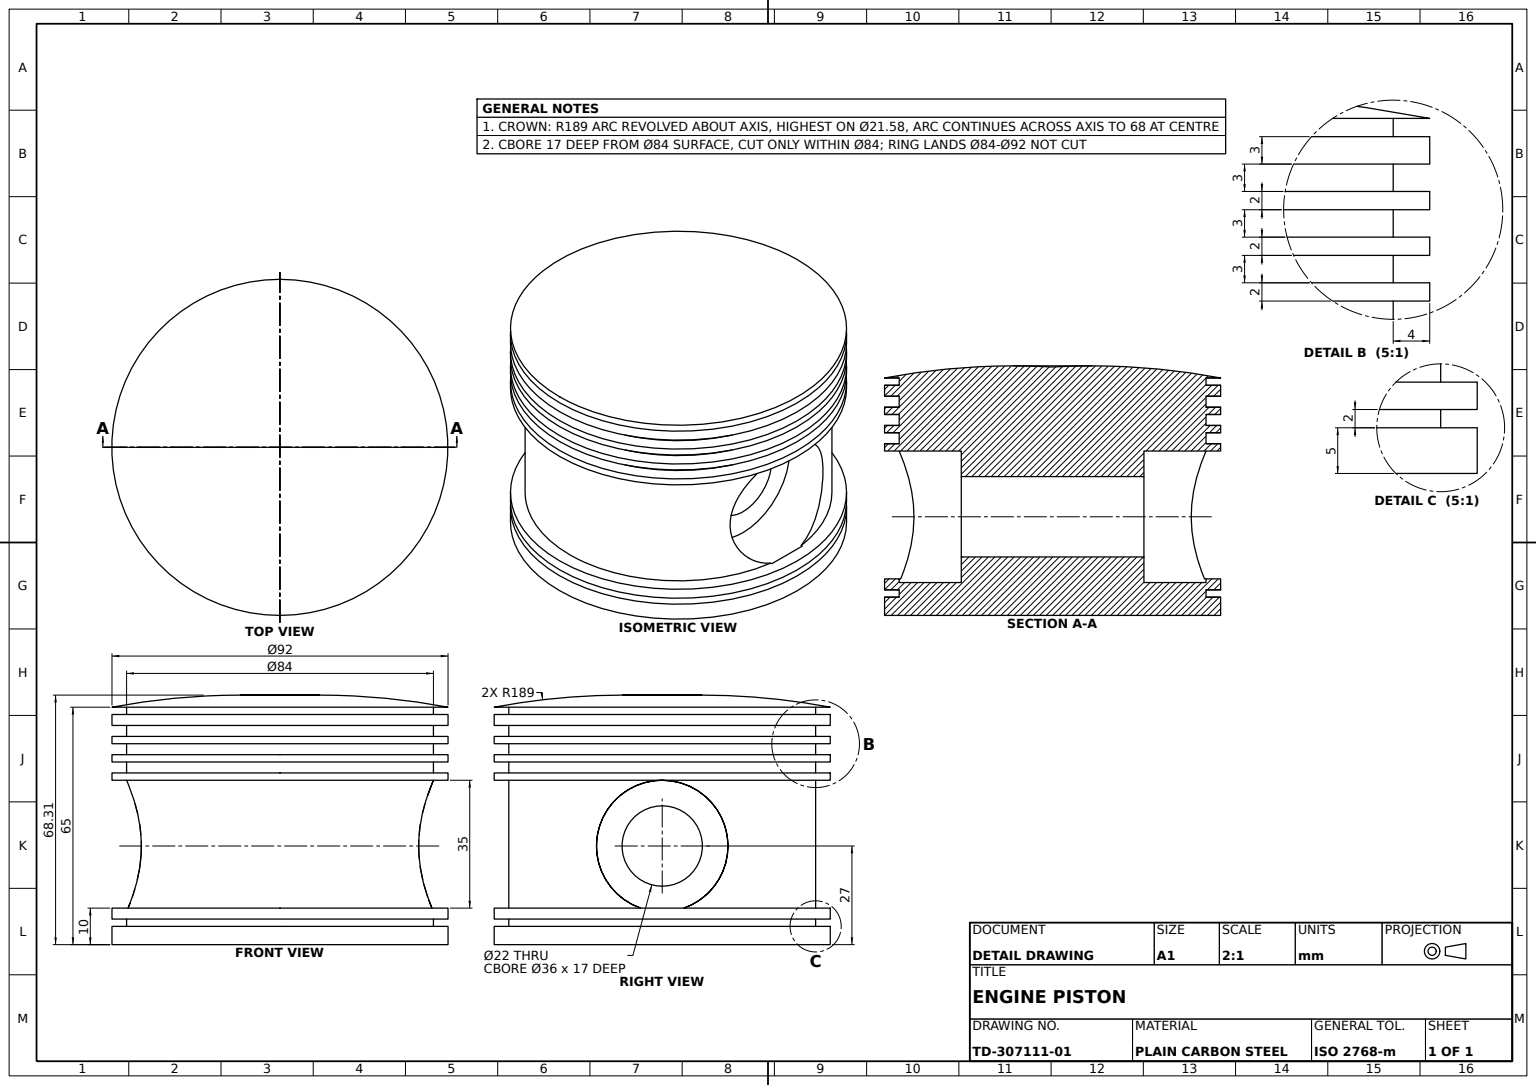
SolidWorks part; units mm, degrees
material "Plain Carbon Steel"
ref_plane "Front Plane" through (0, 0, 0) normal (0, 0, 1) x (1, 0, 0)
ref_plane "Top Plane" through (0, 0, 0) normal (0, 1, 0) x (1, 0, 0)
ref_plane "Right Plane" through (0, 0, 0) normal (1, 0, 0) x (0, 0, -1)
sketch "Piston Profile Sketch" plane through (0, 0, 0) normal (0, 1, 0) x (1, 0, 0)
  line L2 (0, 0) -> (46, 0)
  line L4 (46, 0) -> (46, 5)
  line L5 (46, 5) -> (42, 5)
  line L6 (42, 5) -> (42, 7)
  line L7 (42, 7) -> (46, 7)
  line L8 (46, 7) -> (46, 10)
  line L11 (46, 10) -> (42, 10)
  line L12 (42, 5) -> (42, 7)
  line L13 (42, 10.3777) -> (42, 45)
  line L14 (42, 10) -> (42, 10.3777)
  line L15 (42, 45) -> (46, 45)
  line L16 (46, 45) -> (46, 47)
  line L17 (46, 47) -> (42, 47)
  line L18 (42, 47) -> (42, 50)
  line L19 (42, 50) -> (46, 50)
  line L20 (46, 50) -> (46, 52)
  line L21 (46, 52) -> (42, 52)
  line L22 (42, 52) -> (42, 55)
  line L23 (42, 55) -> (46, 55)
  line L24 (46, 55) -> (46, 57)
  line L25 (46, 57) -> (42, 57)
  line L26 (42, 57) -> (42, 60)
  line L27 (42, 60) -> (46, 60)
  line L28 (46, 60) -> (46, 63)
  line L29 (46, 63) -> (42, 63)
  line L30 (42, 63) -> (42, 65)
  line L31 (0, 0) -> (0, 68)
  line L32 (42, 65) -> (46, 65)
  arc A0 (0, 68) -> (46, 65) centre (10.7918, -120.6916) cw
  point P12 (44, 47)
  point P14 (42, 58.5)
  dimension "D28" = 65
  dimension "D29" = 189
  dimension "D3" = 5
  dimension "D4" = 2
  dimension "D5" = 4
  dimension "D6" = 3
  dimension "D7" = 34.6223
  dimension "D8" = 42
  dimension "D9" = 46
  dimension "D10" = 4
  dimension "D11" = 2
  dimension "D12" = 4
  dimension "D13" = 3
  dimension "D14" = 46
  dimension "D15" = 2
  dimension "D16" = 4
  dimension "D17" = 3
  dimension "D18" = 2
  dimension "D19" = 4
  dimension "D20" = 42
  dimension "D21" = 3
  dimension "D22" = 4
  dimension "D23" = 3
  dimension "D24" = 4
  dimension "D25" = 68
  dimension "D26" = 4
  dimension "D27" = 2
revolve "Piston Body" add sketch "Piston Profile Sketch" angle 360 about L31
ref_plane "Pin Boss Relief Plane" through (0, 42, 0) normal (0, 1, 0) x (1, 0, 0)
sketch "Pin Boss Relief Sketch" plane through (0, 42, 0) normal (0, 1, 0) x (1, 0, 0)
  line L0 (46, 5) -> (-46, 5) construction
  circle A0 centre (0, 27) radius 18
  dimension "D1" = 36
  dimension "D2" = 22
extrude "Pin Boss Relief Ø36" cut sketch "Pin Boss Relief Sketch" against normal blind 17
mirror "Pin Boss Relief Mirror" about plane through (0, 0, 0) normal (0, 1, 0) of "Pin Boss Relief Ø36"
sketch "Wrist Pin Bore Sketch" plane through (0, 25, 0) normal (0, 1, 0) x (1, 0, 0)
  circle A0 centre (0, 27) radius 11
  dimension "D1" = 22
extrude "Wrist Pin Bore" cut sketch "Wrist Pin Bore Sketch" against normal blind 157
